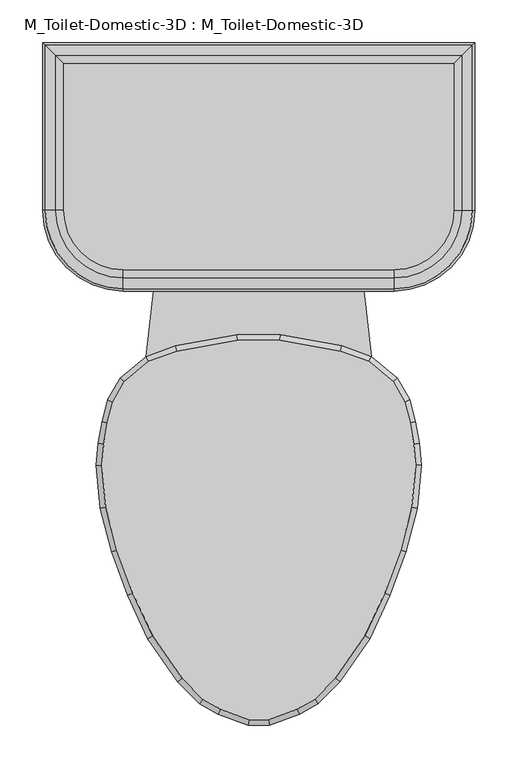
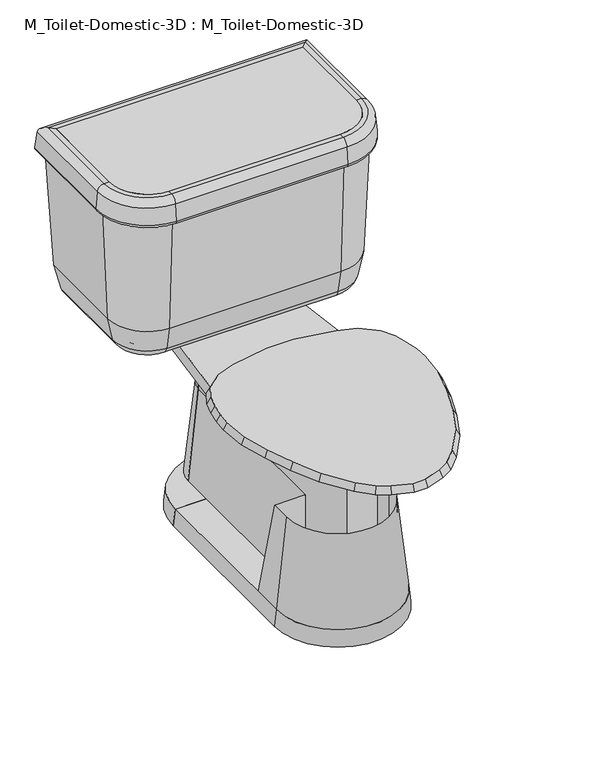
"""IFC4 building model written with IfcOpenShell, lengths in millimetres: flow terminal geometry, M_Toilet-Domestic-3D : M_Toilet-Domestic-3D."""

from ifc_helpers import new_model, si_unit, point, frame, frame_2d, origin, place, context, project, spatial, polyline, circle_curve, ellipse_curve, trimmed, segment, composite_curve, outline, extrude, faceted_brep, source, transform, mapped, element, save
from ifc_brep_helpers import plane_surface, cylinder_surface, revolved_surface, advanced_brep


def m_toilet_domestic_3d_m_toilet_domestic_3d_5cb52bd4(model_context):
    return source(origin(), model_context, "Body", "SolidModel", [
        advanced_brep(
        [(-117.7636364, 285.75, 0.0), (-38.1, 285.75, 0.0), (-38.1, 285.75, 31.75), (-114.3, 285.75, 31.75), (117.7636364, 285.75, 0.0), (114.3, 285.75, 31.75), (38.1, 285.75, 31.75), (38.1, 285.75, 0.0)],
        [
            (0, 1),
            (1, 2),
            (2, 3),
            (3, 0),
            (4, 5),
            (5, 6),
            (6, 7),
            (7, 4),
            (7, 1, circle_curve(frame((0.0, 285.75, 0.0), z_axis=(0.0, 0.0, 1.0), x_axis=(-1.0, 0.0, 0.0)), 38.1)),
            (0, 4, circle_curve(frame((0.0, 285.75, 0.0), z_axis=(0.0, 0.0, -1.0), x_axis=(-1.0, 0.0, 0.0)), 117.7636364)),
            (6, 2, circle_curve(frame((0.0, 285.75, 31.75), z_axis=(0.0, 0.0, 1.0), x_axis=(-1.0, 0.0, 0.0)), 38.1)),
            (5, 3, circle_curve(frame((0.0, 285.75, 31.75), z_axis=(0.0, 0.0, 1.0), x_axis=(-1.0, 0.0, 0.0)), 114.3)),
        ],
        [
            plane_surface(frame((0.0, 285.75, -304.8), z_axis=(0.0, -1.0, 0.0), x_axis=(-1.0, 0.0, 0.0))),
            plane_surface(frame((0.0, 285.75, -304.8), z_axis=(0.0, -1.0, 0.0), x_axis=(1.0, 0.0, 0.0))),
            plane_surface(frame((0.0, 285.75, 0.0), z_axis=(0.0, 0.0, -1.0), x_axis=(-1.0, 0.0, 0.0))),
            revolved_surface(polyline([(-38.1, 285.75, 0.0), (-38.1, 285.75, 31.75)]), (0.0, 285.75, -304.8), (0.0, 0.0, -1.0)),
            plane_surface(frame((0.0, 285.75, 31.75), z_axis=(0.0, 0.0, 1.0), x_axis=(-1.0, 0.0, 0.0))),
            revolved_surface(polyline([(-114.3, 285.75, 31.75), (-117.7636364, 285.75, 0.0)]), (0.0, 285.75, -304.8), (0.0, 0.0, -1.0)),
        ],
        [
            (0, [[1, 2, 3, 4]]),
            (1, [[5, 6, 7, 8]]),
            (2, [[9, -1, 10, -8]]),
            (3, [[11, -2, -9, -7]]),
            (4, [[12, -3, -11, -6]]),
            (5, [[-10, -4, -12, -5]]),
        ],
    ),
        advanced_brep(
        [(-38.1, 342.9, 206.375), (-57.15, 342.9, 31.75), (-38.1, 342.9, 31.75), (38.1, 342.9, 206.375), (38.1, 342.9, 31.75), (57.15, 342.9, 31.75)],
        [
            (0, 1),
            (1, 2),
            (2, 0),
            (3, 4),
            (4, 5),
            (5, 3),
            (5, 1, circle_curve(frame((0.0, 342.9, 31.75), z_axis=(0.0, 0.0, 1.0), x_axis=(-1.0, 0.0, 0.0)), 57.15)),
            (0, 3, circle_curve(frame((0.0, 342.9, 206.375), z_axis=(0.0, 0.0, -1.0), x_axis=(-1.0, 0.0, 0.0)), 38.1)),
            (4, 2, circle_curve(frame((0.0, 342.9, 31.75), z_axis=(0.0, 0.0, 1.0), x_axis=(-1.0, 0.0, 0.0)), 38.1)),
        ],
        [
            plane_surface(frame((0.0, 342.9, 31.75), z_axis=(0.0, -1.0, 0.0), x_axis=(-1.0, 0.0, 0.0))),
            plane_surface(frame((0.0, 342.9, 31.75), z_axis=(0.0, -1.0, 0.0), x_axis=(1.0, 0.0, 0.0))),
            revolved_surface(polyline([(-38.1, 342.9, 206.375), (-57.15, 342.9, 31.75)]), (0.0, 342.9, 31.75), (0.0, 0.0, -1.0)),
            plane_surface(frame((0.0, 342.9, 31.75), z_axis=(0.0, 0.0, -1.0), x_axis=(-1.0, 0.0, 0.0))),
            revolved_surface(polyline([(-38.1, 342.9, 31.75), (-38.1, 342.9, 206.375)]), (0.0, 342.9, 31.75), (0.0, 0.0, -1.0)),
        ],
        [
            (0, [[1, 2, 3]]),
            (1, [[4, 5, 6]]),
            (2, [[7, -1, 8, -6]]),
            (3, [[9, -2, -7, -5]]),
            (4, [[-8, -3, -9, -4]]),
        ],
    ),
        faceted_brep([(-157.6293435, 97.472128, 400.05), (-171.060664, 73.773864, 400.05), (-177.5851102, 49.4242991, 400.05), (-181.9845715, 24.4737144, 400.05), (-184.125744, 0.0, 400.05), (-179.7950716, -49.4998127, 400.05), (-166.347, -99.688699, 400.05), (-148.0469602, -149.9676451, 400.05), (-124.7045808, -200.0255393, 400.05), (-90.0971582, -249.9125941, 400.05), (-65.691017, -274.3187354, 400.05), (-44.8990862, -286.3229622, 400.05), (-11.5803237, -298.45, 400.05), (11.5803237, -298.45, 400.05), (44.8990862, -286.3229622, 400.05), (65.691017, -274.3187354, 400.05), (90.0971582, -249.9125941, 400.05), (124.7045808, -200.0255393, 400.05), (148.0469602, -149.9676451, 400.05), (166.347, -99.688699, 400.05), (179.7950716, -49.4998127, 400.05), (184.125744, 0.0, 400.05), (181.9845715, 24.4737144, 400.05), (177.5851102, 49.4242991, 400.05), (171.060664, 73.773864, 400.05), (157.6293435, 97.472128, 400.05), (129.0942628, 121.4159037, 400.05), (95.7755003, 133.5429415, 400.05), (24.844447, 146.05, 400.05), (-24.844447, 146.05, 400.05), (-95.7755003, 133.5429415, 400.05), (-129.0942628, 121.4159037, 400.05), (-162.5887836, 101.6, 387.2181453), (-132.3182423, 127.0, 387.2181453), (-97.4252791, 139.7, 387.2181453), (-25.4, 152.4, 387.2181453), (25.4, 152.4, 387.2181453), (97.4252791, 139.7, 387.2181453), (132.3182423, 127.0, 387.2181453), (162.5887836, 101.6, 387.2181453), (176.9845865, 76.2, 387.2181453), (183.790496, 50.8, 387.2181453), (188.2862441, 25.3033453, 387.2181453), (190.5, 0.0, 387.2181453), (186.0724883, -50.6066907, 387.2181453), (172.4088722, -101.6, 387.2181453), (153.9191843, -152.4, 387.2181453), (130.2307553, -203.2, 387.2181453), (94.9900085, -254.0, 387.2181453), (69.5900085, -279.4, 387.2181453), (47.5929632, -292.1, 387.2181453), (12.7, -304.8, 387.2181453), (-12.7, -304.8, 387.2181453), (-47.5929632, -292.1, 387.2181453), (-69.5900085, -279.4, 387.2181453), (-94.9900085, -254.0, 387.2181453), (-130.2307553, -203.2, 387.2181453), (-153.9191843, -152.4, 387.2181453), (-172.4088722, -101.6, 387.2181453), (-186.0724883, -50.6066907, 387.2181453), (-190.5, 0.0, 387.2181453), (-188.2862441, 25.3033453, 387.2181453), (-183.790496, 50.8, 387.2181453), (-176.9845865, 76.2, 387.2181453)], [[[0, 1, 2, 3, 4, 5, 6, 7, 8, 9, 10, 11, 12, 13, 14, 15, 16, 17, 18, 19, 20, 21, 22, 23, 24, 25, 26, 27, 28, 29, 30, 31]], [[32, 33, 34, 35, 36, 37, 38, 39, 40, 41, 42, 43, 44, 45, 46, 47, 48, 49, 50, 51, 52, 53, 54, 55, 56, 57, 58, 59, 60, 61, 62, 63]], [[32, 63, 1, 0]], [[63, 62, 2, 1]], [[62, 61, 3, 2]], [[61, 60, 4, 3]], [[60, 59, 5, 4]], [[59, 58, 6, 5]], [[58, 57, 7, 6]], [[57, 56, 8, 7]], [[56, 55, 9, 8]], [[55, 54, 10, 9]], [[54, 53, 11, 10]], [[53, 52, 12, 11]], [[52, 51, 13, 12]], [[51, 50, 14, 13]], [[50, 49, 15, 14]], [[49, 48, 16, 15]], [[48, 47, 17, 16]], [[47, 46, 18, 17]], [[46, 45, 19, 18]], [[45, 44, 20, 19]], [[44, 43, 21, 20]], [[43, 42, 22, 21]], [[42, 41, 23, 22]], [[41, 40, 24, 23]], [[40, 39, 25, 24]], [[39, 38, 26, 25]], [[38, 37, 27, 26]], [[37, 36, 28, 27]], [[36, 35, 29, 28]], [[35, 34, 30, 29]], [[34, 33, 31, 30]], [[33, 32, 0, 31]]]),
        extrude(outline(composite_curve([segment(polyline([(228.5868869, 469.8868869), (228.5868869, 298.45)]), True, "CONTINUOUS"), segment(trimmed(circle_curve(frame_2d((158.75, 298.45)), 69.8368869), [point((228.5868869, 298.45))], [point((158.75, 228.6131131))], False, "CARTESIAN"), True, "CONTINUOUS"), segment(polyline([(158.75, 228.6131131), (-158.75, 228.6131131)]), True, "CONTINUOUS"), segment(trimmed(circle_curve(frame_2d((-158.75, 298.45)), 69.8368869), [point((-158.75, 228.6131131))], [point((-228.5868869, 298.45))], False, "CARTESIAN"), True, "CONTINUOUS"), segment(polyline([(-228.5868869, 298.45), (-228.5868869, 469.8868869), (228.5868869, 469.8868869)]), True, "CONTINUOUS")], self_intersect=False)), frame((0.0, 0.0, 654.05), z_axis=(0.0, 0.0, 1.0), x_axis=(1.0, 0.0, 0.0)), (0.0, 0.0, 1.0), 50.8),
        extrude(outline(composite_curve([segment(trimmed(circle_curve(frame_2d((0.0, 342.9)), 38.1), [point((-38.1, 342.9))], [point((38.1, 342.9))], False, "CARTESIAN"), True, "CONTINUOUS"), segment(polyline([(38.1, 342.9), (-38.1, 342.9)]), True, "CONTINUOUS")], self_intersect=False)), frame((0.0, 0.0, 206.375), z_axis=(0.0, 0.0, 1.0), x_axis=(1.0, 0.0, 0.0)), (0.0, 0.0, 1.0), 130.175),
        advanced_brep(
        [(177.8, 419.1, 387.2181453), (177.8, 419.1, 374.65), (177.8, 298.45, 374.65), (177.8, 298.45, 387.2181453), (192.8020829, 434.1020829, 387.2181453), (192.8020829, 298.45, 387.2181453), (211.4650931, 452.7650931, 402.4478636), (211.4650931, 298.45, 402.4478636), (218.7732506, 460.0732506, 438.15), (218.7732506, 298.45, 438.15), (228.5868869, 469.8868869, 654.05), (228.5868869, 298.45, 654.05), (228.5868869, 469.8868869, 704.85), (228.5868869, 298.45, 704.85), (237.91817, 479.21817, 704.85), (237.91817, 298.45, 704.85), (250.5698426, 491.8698426, 693.2568779), (250.5698426, 298.45, 693.2568779), (253.3960274, 494.6960274, 660.953439), (253.3960274, 298.45, 660.953439), (247.070191, 488.370191, 654.05), (247.070191, 298.45, 654.05), (241.3, 482.6, 654.05), (241.3, 298.45, 654.05), (231.4863636, 472.7863636, 438.15), (231.4863636, 298.45, 438.15), (222.3416824, 463.6416824, 393.4759963), (222.3416824, 298.45, 393.4759963), (197.8071664, 439.1071664, 374.65), (197.8071664, 298.45, 374.65), (158.75, 279.4, 387.2181453), (158.75, 279.4, 374.65), (158.75, 264.3979171, 387.2181453), (158.75, 245.7349069, 402.4478636), (158.75, 238.4267494, 438.15), (158.75, 228.6131131, 654.05), (158.75, 228.6131131, 704.85), (158.75, 219.28183, 704.85), (158.75, 206.6301574, 693.2568779), (158.75, 203.8039726, 660.953439), (158.75, 210.129809, 654.05), (158.75, 215.9, 654.05), (158.75, 225.7136364, 438.15), (158.75, 234.8583176, 393.4759963), (158.75, 259.3928336, 374.65), (-158.75, 279.4, 374.65), (-158.75, 279.4, 387.2181453), (-158.75, 264.3979171, 387.2181453), (-158.75, 245.7349069, 402.4478636), (-158.75, 238.4267494, 438.15), (-158.75, 228.6131131, 654.05), (-158.75, 228.6131131, 704.85), (-158.75, 219.28183, 704.85), (-158.75, 206.6301574, 693.2568779), (-158.75, 203.8039726, 660.953439), (-158.75, 210.129809, 654.05), (-158.75, 215.9, 654.05), (-158.75, 225.7136364, 438.15), (-158.75, 234.8583176, 393.4759963), (-158.75, 259.3928336, 374.65), (-177.8, 298.45, 387.2181453), (-177.8, 298.45, 374.65), (-192.8020829, 298.45, 387.2181453), (-211.4650931, 298.45, 402.4478636), (-218.7732506, 298.45, 438.15), (-228.5868869, 298.45, 654.05), (-228.5868869, 298.45, 704.85), (-237.91817, 298.45, 704.85), (-250.5698426, 298.45, 693.2568779), (-253.3960274, 298.45, 660.953439), (-247.070191, 298.45, 654.05), (-241.3, 298.45, 654.05), (-231.4863636, 298.45, 438.15), (-222.3416824, 298.45, 393.4759963), (-197.8071664, 298.45, 374.65), (-177.8, 419.1, 374.65), (-177.8, 419.1, 387.2181453), (-192.8020829, 434.1020829, 387.2181453), (-211.4650931, 452.7650931, 402.4478636), (-218.7732506, 460.0732506, 438.15), (-228.5868869, 469.8868869, 654.05), (-228.5868869, 469.8868869, 704.85), (-237.91817, 479.21817, 704.85), (-250.5698426, 491.8698426, 693.2568779), (-253.3960274, 494.6960274, 660.953439), (-247.070191, 488.370191, 654.05), (-241.3, 482.6, 654.05), (-231.4863636, 472.7863636, 438.15), (-222.3416824, 463.6416824, 393.4759963), (-197.8071664, 439.1071664, 374.65)],
        [
            (0, 1),
            (1, 2),
            (2, 3),
            (3, 0),
            (4, 0),
            (3, 5),
            (5, 4),
            (6, 4, ellipse_curve(frame((192.8020829, 434.1020829, 406.2681453), z_axis=(-0.7071067811865451, 0.7071067811865498, 0.0), x_axis=(-0.7071067811865497, -0.7071067811865452, 0.0)), 26.9407684, 19.05)),
            (5, 7, circle_curve(frame((192.8020829, 298.45, 406.2681453), z_axis=(0.0, -1.0, 0.0), x_axis=(1.0, 0.0, 0.0)), 19.05)),
            (7, 6),
            (8, 6),
            (7, 9),
            (9, 8),
            (10, 8),
            (9, 11),
            (11, 10),
            (12, 10),
            (11, 13),
            (13, 12),
            (14, 12),
            (13, 15),
            (15, 14),
            (16, 14, ellipse_curve(frame((237.91817, 479.21817, 692.15), z_axis=(0.7071067811865451, -0.7071067811865498, 0.0), x_axis=(0.7071067811865497, 0.7071067811865452, 0.0)), 17.9605122, 12.7)),
            (15, 17, circle_curve(frame((237.91817, 298.45, 692.15), z_axis=(0.0, 1.0, 0.0), x_axis=(1.0, 0.0, 0.0)), 12.7)),
            (17, 16),
            (18, 16),
            (17, 19),
            (19, 18),
            (20, 18, ellipse_curve(frame((247.070191, 488.370191, 660.4), z_axis=(0.7071067811865451, -0.7071067811865498, 0.0), x_axis=(0.7071067811865497, 0.7071067811865452, 0.0)), 8.9802561, 6.35)),
            (19, 21, circle_curve(frame((247.070191, 298.45, 660.4), z_axis=(0.0, 1.0, 0.0), x_axis=(1.0, 0.0, 0.0)), 6.35)),
            (21, 20),
            (22, 20),
            (21, 23),
            (23, 22),
            (24, 22),
            (23, 25),
            (25, 24),
            (26, 24),
            (25, 27),
            (27, 26),
            (28, 26, ellipse_curve(frame((197.8071664, 439.1071664, 400.05), z_axis=(0.7071067811865451, -0.7071067811865498, 0.0), x_axis=(0.7071067811865497, 0.7071067811865452, 0.0)), 35.9210245, 25.4)),
            (27, 29, circle_curve(frame((197.8071664, 298.45, 400.05), z_axis=(0.0, 1.0, 0.0), x_axis=(1.0, 0.0, 0.0)), 25.4)),
            (29, 28),
            (1, 28),
            (29, 2),
            (30, 3, circle_curve(frame((158.75, 298.45, 387.2181453), z_axis=(0.0, 0.0, 1.0), x_axis=(1.0, 0.0, 0.0)), 19.05)),
            (2, 31, circle_curve(frame((158.75, 298.45, 374.65), z_axis=(0.0, 0.0, -1.0), x_axis=(1.0, 0.0, 0.0)), 19.05)),
            (31, 30),
            (32, 5, circle_curve(frame((158.75, 298.45, 387.2181453), z_axis=(0.0, 0.0, 1.0), x_axis=(1.0, 0.0, 0.0)), 34.0520829)),
            (30, 32),
            (33, 7, circle_curve(frame((158.75, 298.45, 402.4478636), z_axis=(0.0, 0.0, 1.0), x_axis=(1.0, 0.0, 0.0)), 52.7150931)),
            (32, 33, circle_curve(frame((158.75, 264.3979171, 406.2681453), z_axis=(-1.0, 0.0, 0.0), x_axis=(0.0, -1.0, 0.0)), 19.05)),
            (34, 9, circle_curve(frame((158.75, 298.45, 438.15), z_axis=(0.0, 0.0, 1.0), x_axis=(1.0, 0.0, 0.0)), 60.0232506)),
            (33, 34),
            (35, 11, circle_curve(frame((158.75, 298.45, 654.05), z_axis=(0.0, 0.0, 1.0), x_axis=(1.0, 0.0, 0.0)), 69.8368869)),
            (34, 35),
            (36, 13, circle_curve(frame((158.75, 298.45, 704.85), z_axis=(0.0, 0.0, 1.0), x_axis=(1.0, 0.0, 0.0)), 69.8368869)),
            (35, 36),
            (37, 15, circle_curve(frame((158.75, 298.45, 704.85), z_axis=(0.0, 0.0, 1.0), x_axis=(1.0, 0.0, 0.0)), 79.16817)),
            (36, 37),
            (38, 17, circle_curve(frame((158.75, 298.45, 693.2568779), z_axis=(0.0, 0.0, 1.0), x_axis=(1.0, 0.0, 0.0)), 91.8198426)),
            (37, 38, circle_curve(frame((158.75, 219.28183, 692.15), z_axis=(1.0, 0.0, 0.0), x_axis=(0.0, -1.0, 0.0)), 12.7)),
            (39, 19, circle_curve(frame((158.75, 298.45, 660.953439), z_axis=(0.0, 0.0, 1.0), x_axis=(1.0, 0.0, 0.0)), 94.6460274)),
            (38, 39),
            (40, 21, circle_curve(frame((158.75, 298.45, 654.05), z_axis=(0.0, 0.0, 1.0), x_axis=(1.0, 0.0, 0.0)), 88.320191)),
            (39, 40, circle_curve(frame((158.75, 210.129809, 660.4), z_axis=(1.0, 0.0, 0.0), x_axis=(0.0, -1.0, 0.0)), 6.35)),
            (41, 23, circle_curve(frame((158.75, 298.45, 654.05), z_axis=(0.0, 0.0, 1.0), x_axis=(1.0, 0.0, 0.0)), 82.55)),
            (40, 41),
            (42, 25, circle_curve(frame((158.75, 298.45, 438.15), z_axis=(0.0, 0.0, 1.0), x_axis=(1.0, 0.0, 0.0)), 72.7363636)),
            (41, 42),
            (43, 27, circle_curve(frame((158.75, 298.45, 393.4759963), z_axis=(0.0, 0.0, 1.0), x_axis=(1.0, 0.0, 0.0)), 63.5916824)),
            (42, 43),
            (44, 29, circle_curve(frame((158.75, 298.45, 374.65), z_axis=(0.0, 0.0, 1.0), x_axis=(1.0, 0.0, 0.0)), 39.0571664)),
            (43, 44, circle_curve(frame((158.75, 259.3928336, 400.05), z_axis=(1.0, 0.0, 0.0), x_axis=(0.0, -1.0, 0.0)), 25.4)),
            (44, 31),
            (31, 45),
            (45, 46),
            (46, 30),
            (46, 47),
            (47, 32),
            (47, 48, circle_curve(frame((-158.75, 264.3979171, 406.2681453), z_axis=(-1.0, 0.0, 0.0), x_axis=(0.0, -1.0, 0.0)), 19.05)),
            (48, 33),
            (48, 49),
            (49, 34),
            (49, 50),
            (50, 35),
            (50, 51),
            (51, 36),
            (51, 52),
            (52, 37),
            (52, 53, circle_curve(frame((-158.75, 219.28183, 692.15), z_axis=(1.0, 0.0, 0.0), x_axis=(0.0, -1.0, 0.0)), 12.7)),
            (53, 38),
            (53, 54),
            (54, 39),
            (54, 55, circle_curve(frame((-158.75, 210.129809, 660.4), z_axis=(1.0, 0.0, 0.0), x_axis=(0.0, -1.0, 0.0)), 6.35)),
            (55, 40),
            (55, 56),
            (56, 41),
            (56, 57),
            (57, 42),
            (57, 58),
            (58, 43),
            (58, 59, circle_curve(frame((-158.75, 259.3928336, 400.05), z_axis=(1.0, 0.0, 0.0), x_axis=(0.0, -1.0, 0.0)), 25.4)),
            (59, 44),
            (59, 45),
            (60, 46, circle_curve(frame((-158.75, 298.45, 387.2181453), z_axis=(0.0, 0.0, 1.0), x_axis=(0.0, -1.0, 0.0)), 19.05)),
            (45, 61, circle_curve(frame((-158.75, 298.45, 374.65), z_axis=(0.0, 0.0, -1.0), x_axis=(0.0, -1.0, 0.0)), 19.05)),
            (61, 60),
            (62, 47, circle_curve(frame((-158.75, 298.45, 387.2181453), z_axis=(0.0, 0.0, 1.0), x_axis=(0.0, -1.0, 0.0)), 34.0520829)),
            (60, 62),
            (63, 48, circle_curve(frame((-158.75, 298.45, 402.4478636), z_axis=(0.0, 0.0, 1.0), x_axis=(0.0, -1.0, 0.0)), 52.7150931)),
            (62, 63, circle_curve(frame((-192.8020829, 298.45, 406.2681453), z_axis=(0.0, 1.0, 0.0), x_axis=(-1.0, 0.0, 0.0)), 19.05)),
            (64, 49, circle_curve(frame((-158.75, 298.45, 438.15), z_axis=(0.0, 0.0, 1.0), x_axis=(0.0, -1.0, 0.0)), 60.0232506)),
            (63, 64),
            (65, 50, circle_curve(frame((-158.75, 298.45, 654.05), z_axis=(0.0, 0.0, 1.0), x_axis=(0.0, -1.0, 0.0)), 69.8368869)),
            (64, 65),
            (66, 51, circle_curve(frame((-158.75, 298.45, 704.85), z_axis=(0.0, 0.0, 1.0), x_axis=(0.0, -1.0, 0.0)), 69.8368869)),
            (65, 66),
            (67, 52, circle_curve(frame((-158.75, 298.45, 704.85), z_axis=(0.0, 0.0, 1.0), x_axis=(0.0, -1.0, 0.0)), 79.16817)),
            (66, 67),
            (68, 53, circle_curve(frame((-158.75, 298.45, 693.2568779), z_axis=(0.0, 0.0, 1.0), x_axis=(0.0, -1.0, 0.0)), 91.8198426)),
            (67, 68, circle_curve(frame((-237.91817, 298.45, 692.15), z_axis=(0.0, -1.0, 0.0), x_axis=(-1.0, 0.0, 0.0)), 12.7)),
            (69, 54, circle_curve(frame((-158.75, 298.45, 660.953439), z_axis=(0.0, 0.0, 1.0), x_axis=(0.0, -1.0, 0.0)), 94.6460274)),
            (68, 69),
            (70, 55, circle_curve(frame((-158.75, 298.45, 654.05), z_axis=(0.0, 0.0, 1.0), x_axis=(0.0, -1.0, 0.0)), 88.320191)),
            (69, 70, circle_curve(frame((-247.070191, 298.45, 660.4), z_axis=(0.0, -1.0, 0.0), x_axis=(-1.0, 0.0, 0.0)), 6.35)),
            (71, 56, circle_curve(frame((-158.75, 298.45, 654.05), z_axis=(0.0, 0.0, 1.0), x_axis=(0.0, -1.0, 0.0)), 82.55)),
            (70, 71),
            (72, 57, circle_curve(frame((-158.75, 298.45, 438.15), z_axis=(0.0, 0.0, 1.0), x_axis=(0.0, -1.0, 0.0)), 72.7363636)),
            (71, 72),
            (73, 58, circle_curve(frame((-158.75, 298.45, 393.4759963), z_axis=(0.0, 0.0, 1.0), x_axis=(0.0, -1.0, 0.0)), 63.5916824)),
            (72, 73),
            (74, 59, circle_curve(frame((-158.75, 298.45, 374.65), z_axis=(0.0, 0.0, 1.0), x_axis=(0.0, -1.0, 0.0)), 39.0571664)),
            (73, 74, circle_curve(frame((-197.8071664, 298.45, 400.05), z_axis=(0.0, -1.0, 0.0), x_axis=(-1.0, 0.0, 0.0)), 25.4)),
            (74, 61),
            (61, 75),
            (75, 76),
            (76, 60),
            (76, 77),
            (77, 62),
            (77, 78, ellipse_curve(frame((-192.8020829, 434.1020829, 406.2681453), z_axis=(0.7071067811865498, 0.7071067811865451, 0.0), x_axis=(-0.7071067811865451, 0.70710678118655, 0.0)), 26.9407684, 19.05)),
            (78, 63),
            (78, 79),
            (79, 64),
            (79, 80),
            (80, 65),
            (80, 81),
            (81, 66),
            (81, 82),
            (82, 67),
            (82, 83, ellipse_curve(frame((-237.91817, 479.21817, 692.15), z_axis=(-0.7071067811865498, -0.7071067811865451, 0.0), x_axis=(0.7071067811865451, -0.70710678118655, 0.0)), 17.9605122, 12.7)),
            (83, 68),
            (83, 84),
            (84, 69),
            (84, 85, ellipse_curve(frame((-247.070191, 488.370191, 660.4), z_axis=(-0.7071067811865498, -0.7071067811865451, 0.0), x_axis=(0.7071067811865451, -0.70710678118655, 0.0)), 8.9802561, 6.35)),
            (85, 70),
            (85, 86),
            (86, 71),
            (86, 87),
            (87, 72),
            (87, 88),
            (88, 73),
            (88, 89, ellipse_curve(frame((-197.8071664, 439.1071664, 400.05), z_axis=(-0.7071067811865498, -0.7071067811865451, 0.0), x_axis=(0.7071067811865451, -0.70710678118655, 0.0)), 35.9210245, 25.4)),
            (89, 74),
            (89, 75),
            (75, 1),
            (0, 76),
            (4, 77),
            (6, 78),
            (8, 79),
            (10, 80),
            (12, 81),
            (14, 82),
            (16, 83),
            (18, 84),
            (20, 85),
            (22, 86),
            (24, 87),
            (26, 88),
            (28, 89),
        ],
        [
            plane_surface(frame((177.8, 419.1, 374.65), z_axis=(-1.0, 0.0, 0.0), x_axis=(0.0, -1.0, 0.0))),
            plane_surface(frame((177.8, 419.1, 387.2181453), z_axis=(0.0, 0.0, 1.0), x_axis=(0.0, -1.0, 0.0))),
            revolved_surface(polyline([(211.8520829, 298.45, 406.2681453), (211.8520829, 453.1520829260162, 406.2681453)]), (192.8020829, 419.1, 406.2681453), (0.0, -1.0, 0.0)),
            plane_surface(frame((211.4650931, 452.7650931, 402.4478636), z_axis=(-0.9796855721787505, 0.0, 0.2005397209153197), x_axis=(0.0, -1.0, 0.0))),
            plane_surface(frame((218.7732506, 460.0732506, 438.15), z_axis=(-0.9989685402102993, 0.0, 0.04540766091865541), x_axis=(0.0, -1.0, 0.0))),
            plane_surface(frame((228.5868869, 469.8868869, 654.05), z_axis=(-1.0, 0.0, 0.0), x_axis=(0.0, -1.0, 0.0))),
            plane_surface(frame((228.5868869, 469.8868869, 704.85), z_axis=(0.0, 0.0, 1.0), x_axis=(0.0, -1.0, 0.0))),
            cylinder_surface(frame((237.91817, 419.1, 692.15), z_axis=(0.0, 1.0, 0.0), x_axis=(1.0, 0.0, 0.0)), 12.7),
            plane_surface(frame((250.5698426, 491.8698426, 693.2568779), z_axis=(0.9961946980917448, 0.0, 0.08715574274766702), x_axis=(0.0, -1.0, 0.0))),
            cylinder_surface(frame((247.070191, 419.1, 660.4), z_axis=(0.0, 1.0, 0.0), x_axis=(1.0, 0.0, 0.0)), 6.35),
            plane_surface(frame((247.070191, 488.370191, 654.05), z_axis=(0.0, 0.0, -1.0), x_axis=(0.0, -1.0, 0.0))),
            plane_surface(frame((241.3, 482.6, 654.05), z_axis=(0.9989685402102995, 0.0, -0.04540766091865437), x_axis=(0.0, -1.0, 0.0))),
            plane_surface(frame((231.4863636, 472.7863636, 438.15), z_axis=(0.9796855721787479, 0.0, -0.2005397209153326), x_axis=(0.0, -1.0, 0.0))),
            cylinder_surface(frame((197.8071664, 419.1, 400.05), z_axis=(0.0, 1.0, 0.0), x_axis=(1.0, 0.0, 0.0)), 25.4),
            plane_surface(frame((197.8071664, 439.1071664, 374.65), z_axis=(0.0, 0.0, -1.0), x_axis=(0.0, -1.0, 0.0))),
            revolved_surface(polyline([(177.8, 298.45, 374.65), (177.8, 298.45, 387.2181453)]), (158.75, 298.45, 0.0), (0.0, 0.0, -1.0)),
            plane_surface(frame((158.75, 298.45, 387.2181453), z_axis=(0.0, 0.0, 1.0), x_axis=(1.0, 0.0, 0.0))),
            revolved_surface(trimmed(ellipse_curve(frame((192.8020829, 298.45, 406.2681453), z_axis=(0.0, -1.0, 0.0), x_axis=(1.0, 0.0, 0.0)), 19.05, 19.05), [point((192.8020829, 298.45, 387.2181453))], [point((211.4650931, 298.45, 402.4478636))], True, "CARTESIAN"), (158.75, 298.45, 0.0), (0.0, 0.0, -1.0)),
            revolved_surface(polyline([(211.4650931, 298.45, 402.4478636), (218.7732506, 298.45, 438.15)]), (158.75, 298.45, 0.0), (0.0, 0.0, -1.0)),
            revolved_surface(polyline([(218.7732506, 298.45, 438.15), (228.5868869, 298.45, 654.05)]), (158.75, 298.45, 0.0), (0.0, 0.0, -1.0)),
            revolved_surface(polyline([(228.5868869, 298.45, 654.05), (228.5868869, 298.45, 704.85)]), (158.75, 298.45, 0.0), (0.0, 0.0, -1.0)),
            plane_surface(frame((158.75, 298.45, 704.85), z_axis=(0.0, 0.0, 1.0), x_axis=(1.0, 0.0, 0.0))),
            revolved_surface(trimmed(ellipse_curve(frame((237.91817, 298.45, 692.15), z_axis=(0.0, 1.0, 0.0), x_axis=(1.0, 0.0, 0.0)), 12.7, 12.7), [point((237.91817, 298.45, 704.85))], [point((250.5698426, 298.45, 693.2568779))], True, "CARTESIAN"), (158.75, 298.45, 0.0), (0.0, 0.0, -1.0)),
            revolved_surface(polyline([(250.5698426, 298.45, 693.2568779), (253.3960274, 298.45, 660.953439)]), (158.75, 298.45, 0.0), (0.0, 0.0, -1.0)),
            revolved_surface(trimmed(ellipse_curve(frame((247.070191, 298.45, 660.4), z_axis=(0.0, 1.0, 0.0), x_axis=(1.0, 0.0, 0.0)), 6.35, 6.35), [point((253.3960274, 298.45, 660.953439))], [point((247.070191, 298.45, 654.05))], True, "CARTESIAN"), (158.75, 298.45, 0.0), (0.0, 0.0, -1.0)),
            plane_surface(frame((158.75, 298.45, 654.05), z_axis=(0.0, 0.0, -1.0), x_axis=(1.0, 0.0, 0.0))),
            revolved_surface(polyline([(241.3, 298.45, 654.05), (231.4863636, 298.45, 438.15)]), (158.75, 298.45, 0.0), (0.0, 0.0, -1.0)),
            revolved_surface(polyline([(231.4863636, 298.45, 438.15), (222.3416824, 298.45, 393.4759963)]), (158.75, 298.45, 0.0), (0.0, 0.0, -1.0)),
            revolved_surface(trimmed(ellipse_curve(frame((197.8071664, 298.45, 400.05), z_axis=(0.0, 1.0, 0.0), x_axis=(1.0, 0.0, 0.0)), 25.4, 25.4), [point((222.3416824, 298.45, 393.4759963))], [point((197.8071664, 298.45, 374.65))], True, "CARTESIAN"), (158.75, 298.45, 0.0), (0.0, 0.0, -1.0)),
            plane_surface(frame((158.75, 298.45, 374.65), z_axis=(0.0, 0.0, -1.0), x_axis=(1.0, 0.0, 0.0))),
            plane_surface(frame((158.75, 279.4, 374.65), z_axis=(0.0, 1.0, 0.0), x_axis=(-1.0, 0.0, 0.0))),
            plane_surface(frame((158.75, 279.4, 387.2181453), z_axis=(0.0, 0.0, 1.0), x_axis=(-1.0, 0.0, 0.0))),
            revolved_surface(polyline([(-158.75, 245.34791709999996, 406.2681453), (158.75, 245.34791709999996, 406.2681453)]), (158.75, 264.3979171, 406.2681453), (-1.0, 0.0, 0.0)),
            plane_surface(frame((158.75, 245.7349069, 402.4478636), z_axis=(0.0, 0.9796855721787505, 0.2005397209153197), x_axis=(-1.0, 0.0, 0.0))),
            plane_surface(frame((158.75, 238.4267494, 438.15), z_axis=(0.0, 0.9989685402102993, 0.04540766091865541), x_axis=(-1.0, 0.0, 0.0))),
            plane_surface(frame((158.75, 228.6131131, 654.05), z_axis=(0.0, 1.0, 0.0), x_axis=(-1.0, 0.0, 0.0))),
            plane_surface(frame((158.75, 228.6131131, 704.85), z_axis=(0.0, 0.0, 1.0), x_axis=(-1.0, 0.0, 0.0))),
            cylinder_surface(frame((158.75, 219.28183, 692.15), z_axis=(1.0, 0.0, 0.0), x_axis=(0.0, -1.0, 0.0)), 12.7),
            plane_surface(frame((158.75, 206.6301574, 693.2568779), z_axis=(0.0, -0.9961946980917448, 0.08715574274766702), x_axis=(-1.0, 0.0, 0.0))),
            cylinder_surface(frame((158.75, 210.129809, 660.4), z_axis=(1.0, 0.0, 0.0), x_axis=(0.0, -1.0, 0.0)), 6.35),
            plane_surface(frame((158.75, 210.129809, 654.05), z_axis=(0.0, 0.0, -1.0), x_axis=(-1.0, 0.0, 0.0))),
            plane_surface(frame((158.75, 215.9, 654.05), z_axis=(0.0, -0.9989685402102995, -0.04540766091865437), x_axis=(-1.0, 0.0, 0.0))),
            plane_surface(frame((158.75, 225.7136364, 438.15), z_axis=(0.0, -0.9796855721787479, -0.2005397209153326), x_axis=(-1.0, 0.0, 0.0))),
            cylinder_surface(frame((158.75, 259.3928336, 400.05), z_axis=(1.0, 0.0, 0.0), x_axis=(0.0, -1.0, 0.0)), 25.4),
            plane_surface(frame((158.75, 259.3928336, 374.65), z_axis=(0.0, 0.0, -1.0), x_axis=(-1.0, 0.0, 0.0))),
            revolved_surface(polyline([(-158.75, 279.4, 374.65), (-158.75, 279.4, 387.2181453)]), (-158.75, 298.45, 0.0), (0.0, 0.0, -1.0)),
            plane_surface(frame((-158.75, 298.45, 387.2181453), z_axis=(0.0, 0.0, 1.0), x_axis=(0.0, -1.0, 0.0))),
            revolved_surface(trimmed(ellipse_curve(frame((-158.75, 264.3979171, 406.2681453), z_axis=(-1.0, 0.0, 0.0), x_axis=(0.0, -1.0, 0.0)), 19.05, 19.05), [point((-158.75, 264.3979171, 387.2181453))], [point((-158.75, 245.7349069, 402.4478636))], True, "CARTESIAN"), (-158.75, 298.45, 0.0), (0.0, 0.0, -1.0)),
            revolved_surface(polyline([(-158.75, 245.7349069, 402.4478636), (-158.75, 238.4267494, 438.15)]), (-158.75, 298.45, 0.0), (0.0, 0.0, -1.0)),
            revolved_surface(polyline([(-158.75, 238.4267494, 438.15), (-158.75, 228.6131131, 654.05)]), (-158.75, 298.45, 0.0), (0.0, 0.0, -1.0)),
            revolved_surface(polyline([(-158.75, 228.6131131, 654.05), (-158.75, 228.6131131, 704.85)]), (-158.75, 298.45, 0.0), (0.0, 0.0, -1.0)),
            plane_surface(frame((-158.75, 298.45, 704.85), z_axis=(0.0, 0.0, 1.0), x_axis=(0.0, -1.0, 0.0))),
            revolved_surface(trimmed(ellipse_curve(frame((-158.75, 219.28183, 692.15), z_axis=(1.0, 0.0, 0.0), x_axis=(0.0, -1.0, 0.0)), 12.7, 12.7), [point((-158.75, 219.28183, 704.85))], [point((-158.75, 206.6301574, 693.2568779))], True, "CARTESIAN"), (-158.75, 298.45, 0.0), (0.0, 0.0, -1.0)),
            revolved_surface(polyline([(-158.75, 206.6301574, 693.2568779), (-158.75, 203.8039726, 660.953439)]), (-158.75, 298.45, 0.0), (0.0, 0.0, -1.0)),
            revolved_surface(trimmed(ellipse_curve(frame((-158.75, 210.129809, 660.4), z_axis=(1.0, 0.0, 0.0), x_axis=(0.0, -1.0, 0.0)), 6.35, 6.35), [point((-158.75, 203.8039726, 660.953439))], [point((-158.75, 210.129809, 654.05))], True, "CARTESIAN"), (-158.75, 298.45, 0.0), (0.0, 0.0, -1.0)),
            plane_surface(frame((-158.75, 298.45, 654.05), z_axis=(0.0, 0.0, -1.0), x_axis=(0.0, -1.0, 0.0))),
            revolved_surface(polyline([(-158.75, 215.9, 654.05), (-158.75, 225.7136364, 438.15)]), (-158.75, 298.45, 0.0), (0.0, 0.0, -1.0)),
            revolved_surface(polyline([(-158.75, 225.7136364, 438.15), (-158.75, 234.8583176, 393.4759963)]), (-158.75, 298.45, 0.0), (0.0, 0.0, -1.0)),
            revolved_surface(trimmed(ellipse_curve(frame((-158.75, 259.3928336, 400.05), z_axis=(1.0, 0.0, 0.0), x_axis=(0.0, -1.0, 0.0)), 25.4, 25.4), [point((-158.75, 234.8583176, 393.4759963))], [point((-158.75, 259.3928336, 374.65))], True, "CARTESIAN"), (-158.75, 298.45, 0.0), (0.0, 0.0, -1.0)),
            plane_surface(frame((-158.75, 298.45, 374.65), z_axis=(0.0, 0.0, -1.0), x_axis=(0.0, -1.0, 0.0))),
            plane_surface(frame((-177.8, 298.45, 374.65), z_axis=(1.0, 0.0, 0.0), x_axis=(0.0, 1.0, 0.0))),
            plane_surface(frame((-177.8, 298.45, 387.2181453), z_axis=(0.0, 0.0, 1.0), x_axis=(0.0, 1.0, 0.0))),
            revolved_surface(polyline([(-211.8520829, 453.15208292601636, 406.2681453), (-211.8520829, 298.45, 406.2681453)]), (-192.8020829, 298.45, 406.2681453), (0.0, 1.0, 0.0)),
            plane_surface(frame((-211.4650931, 298.45, 402.4478636), z_axis=(0.9796855721787505, 0.0, 0.2005397209153197), x_axis=(0.0, 1.0, 0.0))),
            plane_surface(frame((-218.7732506, 298.45, 438.15), z_axis=(0.9989685402102993, 0.0, 0.04540766091865541), x_axis=(0.0, 1.0, 0.0))),
            plane_surface(frame((-228.5868869, 298.45, 654.05), z_axis=(1.0, 0.0, 0.0), x_axis=(0.0, 1.0, 0.0))),
            plane_surface(frame((-228.5868869, 298.45, 704.85), z_axis=(0.0, 0.0, 1.0), x_axis=(0.0, 1.0, 0.0))),
            cylinder_surface(frame((-237.91817, 298.45, 692.15), z_axis=(0.0, -1.0, 0.0), x_axis=(-1.0, 0.0, 0.0)), 12.7),
            plane_surface(frame((-250.5698426, 298.45, 693.2568779), z_axis=(-0.9961946980917448, 0.0, 0.08715574274766702), x_axis=(0.0, 1.0, 0.0))),
            cylinder_surface(frame((-247.070191, 298.45, 660.4), z_axis=(0.0, -1.0, 0.0), x_axis=(-1.0, 0.0, 0.0)), 6.35),
            plane_surface(frame((-247.070191, 298.45, 654.05), z_axis=(0.0, 0.0, -1.0), x_axis=(0.0, 1.0, 0.0))),
            plane_surface(frame((-241.3, 298.45, 654.05), z_axis=(-0.9989685402102995, 0.0, -0.04540766091865437), x_axis=(0.0, 1.0, 0.0))),
            plane_surface(frame((-231.4863636, 298.45, 438.15), z_axis=(-0.9796855721787479, 0.0, -0.2005397209153326), x_axis=(0.0, 1.0, 0.0))),
            cylinder_surface(frame((-197.8071664, 298.45, 400.05), z_axis=(0.0, -1.0, 0.0), x_axis=(-1.0, 0.0, 0.0)), 25.4),
            plane_surface(frame((-197.8071664, 298.45, 374.65), z_axis=(0.0, 0.0, -1.0), x_axis=(0.0, 1.0, 0.0))),
            plane_surface(frame((-177.8, 419.1, 374.65), z_axis=(0.0, -1.0, 0.0), x_axis=(1.0, 0.0, 0.0))),
            plane_surface(frame((-177.8, 419.1, 387.2181453), z_axis=(0.0, 0.0, 1.0), x_axis=(1.0, 0.0, 0.0))),
            revolved_surface(polyline([(211.85208292601635, 453.15208290000004, 406.2681453), (-211.85208292601618, 453.15208290000004, 406.2681453)]), (-177.8, 434.1020829, 406.2681453), (1.0, 0.0, 0.0)),
            plane_surface(frame((-211.4650931, 452.7650931, 402.4478636), z_axis=(0.0, -0.9796855721787505, 0.2005397209153197), x_axis=(1.0, 0.0, 0.0))),
            plane_surface(frame((-218.7732506, 460.0732506, 438.15), z_axis=(0.0, -0.9989685402102993, 0.04540766091865541), x_axis=(1.0, 0.0, 0.0))),
            plane_surface(frame((-228.5868869, 469.8868869, 654.05), z_axis=(0.0, -1.0, 0.0), x_axis=(1.0, 0.0, 0.0))),
            plane_surface(frame((-228.5868869, 469.8868869, 704.85), z_axis=(0.0, 0.0, 1.0), x_axis=(1.0, 0.0, 0.0))),
            cylinder_surface(frame((-177.8, 479.21817, 692.15), z_axis=(-1.0, 0.0, 0.0), x_axis=(0.0, 1.0, 0.0)), 12.7),
            plane_surface(frame((-250.5698426, 491.8698426, 693.2568779), z_axis=(0.0, 0.9961946980917448, 0.08715574274766702), x_axis=(1.0, 0.0, 0.0))),
            cylinder_surface(frame((-177.8, 488.370191, 660.4), z_axis=(-1.0, 0.0, 0.0), x_axis=(0.0, 1.0, 0.0)), 6.35),
            plane_surface(frame((-247.070191, 488.370191, 654.05), z_axis=(0.0, 0.0, -1.0), x_axis=(1.0, 0.0, 0.0))),
            plane_surface(frame((-241.3, 482.6, 654.05), z_axis=(0.0, 0.9989685402102995, -0.04540766091865437), x_axis=(1.0, 0.0, 0.0))),
            plane_surface(frame((-231.4863636, 472.7863636, 438.15), z_axis=(0.0, 0.9796855721787479, -0.2005397209153326), x_axis=(1.0, 0.0, 0.0))),
            cylinder_surface(frame((-177.8, 439.1071664, 400.05), z_axis=(-1.0, 0.0, 0.0), x_axis=(0.0, 1.0, 0.0)), 25.4),
            plane_surface(frame((-197.8071664, 439.1071664, 374.65), z_axis=(0.0, 0.0, -1.0), x_axis=(1.0, 0.0, 0.0))),
        ],
        [
            (0, [[1, 2, 3, 4]]),
            (1, [[5, -4, 6, 7]]),
            (2, [[8, -7, 9, 10]]),
            (3, [[11, -10, 12, 13]]),
            (4, [[14, -13, 15, 16]]),
            (5, [[17, -16, 18, 19]]),
            (6, [[20, -19, 21, 22]]),
            (7, [[23, -22, 24, 25]]),
            (8, [[26, -25, 27, 28]]),
            (9, [[29, -28, 30, 31]]),
            (10, [[32, -31, 33, 34]]),
            (11, [[35, -34, 36, 37]]),
            (12, [[38, -37, 39, 40]]),
            (13, [[41, -40, 42, 43]]),
            (14, [[44, -43, 45, -2]]),
            (15, [[46, -3, 47, 48]]),
            (16, [[49, -6, -46, 50]]),
            (17, [[51, -9, -49, 52]]),
            (18, [[53, -12, -51, 54]]),
            (19, [[55, -15, -53, 56]]),
            (20, [[57, -18, -55, 58]]),
            (21, [[59, -21, -57, 60]]),
            (22, [[61, -24, -59, 62]]),
            (23, [[63, -27, -61, 64]]),
            (24, [[65, -30, -63, 66]]),
            (25, [[67, -33, -65, 68]]),
            (26, [[69, -36, -67, 70]]),
            (27, [[71, -39, -69, 72]]),
            (28, [[73, -42, -71, 74]]),
            (29, [[-47, -45, -73, 75]]),
            (30, [[-48, 76, 77, 78]]),
            (31, [[-50, -78, 79, 80]]),
            (32, [[-52, -80, 81, 82]]),
            (33, [[-54, -82, 83, 84]]),
            (34, [[-56, -84, 85, 86]]),
            (35, [[-58, -86, 87, 88]]),
            (36, [[-60, -88, 89, 90]]),
            (37, [[-62, -90, 91, 92]]),
            (38, [[-64, -92, 93, 94]]),
            (39, [[-66, -94, 95, 96]]),
            (40, [[-68, -96, 97, 98]]),
            (41, [[-70, -98, 99, 100]]),
            (42, [[-72, -100, 101, 102]]),
            (43, [[-74, -102, 103, 104]]),
            (44, [[-75, -104, 105, -76]]),
            (45, [[106, -77, 107, 108]]),
            (46, [[109, -79, -106, 110]]),
            (47, [[111, -81, -109, 112]]),
            (48, [[113, -83, -111, 114]]),
            (49, [[115, -85, -113, 116]]),
            (50, [[117, -87, -115, 118]]),
            (51, [[119, -89, -117, 120]]),
            (52, [[121, -91, -119, 122]]),
            (53, [[123, -93, -121, 124]]),
            (54, [[125, -95, -123, 126]]),
            (55, [[127, -97, -125, 128]]),
            (56, [[129, -99, -127, 130]]),
            (57, [[131, -101, -129, 132]]),
            (58, [[133, -103, -131, 134]]),
            (59, [[-107, -105, -133, 135]]),
            (60, [[-108, 136, 137, 138]]),
            (61, [[-110, -138, 139, 140]]),
            (62, [[-112, -140, 141, 142]]),
            (63, [[-114, -142, 143, 144]]),
            (64, [[-116, -144, 145, 146]]),
            (65, [[-118, -146, 147, 148]]),
            (66, [[-120, -148, 149, 150]]),
            (67, [[-122, -150, 151, 152]]),
            (68, [[-124, -152, 153, 154]]),
            (69, [[-126, -154, 155, 156]]),
            (70, [[-128, -156, 157, 158]]),
            (71, [[-130, -158, 159, 160]]),
            (72, [[-132, -160, 161, 162]]),
            (73, [[-134, -162, 163, 164]]),
            (74, [[-135, -164, 165, -136]]),
            (75, [[-137, 166, -1, 167]]),
            (76, [[-139, -167, -5, 168]]),
            (77, [[-141, -168, -8, 169]]),
            (78, [[-143, -169, -11, 170]]),
            (79, [[-145, -170, -14, 171]]),
            (80, [[-147, -171, -17, 172]]),
            (81, [[-149, -172, -20, 173]]),
            (82, [[-151, -173, -23, 174]]),
            (83, [[-153, -174, -26, 175]]),
            (84, [[-155, -175, -29, 176]]),
            (85, [[-157, -176, -32, 177]]),
            (86, [[-159, -177, -35, 178]]),
            (87, [[-161, -178, -38, 179]]),
            (88, [[-163, -179, -41, 180]]),
            (89, [[-165, -180, -44, -166]]),
        ],
    ),
        extrude(outline(composite_curve([segment(polyline([(-25.4, 152.4), (-97.4252791, 139.7), (-132.3182423, 127.0), (-101.4824733, 395.1508638)]), True, "CONTINUOUS"), segment(trimmed(circle_curve(frame_2d((-88.8656197, 393.7)), 12.7), [point((-101.4824733, 395.1508638))], [point((-88.8656197, 406.4))], False, "CARTESIAN"), True, "CONTINUOUS"), segment(polyline([(-88.8656197, 406.4), (88.8656197, 406.4)]), True, "CONTINUOUS"), segment(trimmed(circle_curve(frame_2d((88.8656197, 393.7)), 12.7), [point((88.8656197, 406.4))], [point((101.4824733, 395.1508638))], False, "CARTESIAN"), True, "CONTINUOUS"), segment(polyline([(101.4824733, 395.1508638), (132.3182423, 127.0), (97.4252791, 139.7), (25.4, 152.4), (0.0, 152.4), (-25.4, 152.4)]), True, "CONTINUOUS")], self_intersect=False)), frame((0.0, 0.0, 336.55), z_axis=(0.0, 0.0, 1.0), x_axis=(1.0, 0.0, 0.0)), (0.0, 0.0, 1.0), 25.4),
        extrude(outline(polyline([(139.7, 264.5247209), (152.4, 336.55), (342.9, 336.55), (342.9, 206.375), (107.4852632, 206.375), (127.0, 229.6317577), (139.7, 264.5247209)])), frame((-38.1, 0.0, 0.0), z_axis=(1.0, 0.0, 0.0), x_axis=(0.0, 1.0, 0.0)), (0.0, 0.0, 1.0), 76.2),
        advanced_brep(
        [(-117.7636364, 285.75, 0.0), (-114.3, 285.75, 31.75), (-38.1, 285.75, 31.75), (-38.1, 285.75, 0.0), (-117.7636364, -38.0999951, 0.0), (-114.3, -38.0999951, 31.75), (-38.1, -38.0999951, 31.75), (-38.1, -38.0999951, 0.0), (114.2999707, -38.0999951, 31.75), (117.7636071, -38.0999951, 0.0), (38.0999707, -38.0999951, 31.75), (38.0999707, -38.0999951, 0.0), (117.7636071, 285.6681634, 0.0), (38.0999707, 285.6681634, 0.0), (38.0999707, 285.6681634, 31.75), (114.2999707, 285.6681634, 31.75)],
        [
            (0, 1),
            (1, 2),
            (2, 3),
            (3, 0),
            (0, 4),
            (4, 5),
            (5, 1),
            (5, 6),
            (6, 2),
            (6, 7),
            (7, 3),
            (7, 4),
            (8, 5, circle_curve(frame((-1.46e-05, -38.0999951, 31.75), z_axis=(0.0, 0.0, -1.0), x_axis=(-1.0, 0.0, 0.0)), 114.2999854)),
            (4, 9, circle_curve(frame((-1.46e-05, -38.0999951, 0.0), z_axis=(0.0, 0.0, 1.0), x_axis=(-1.0, 0.0, 0.0)), 117.7636217)),
            (9, 8),
            (10, 6, circle_curve(frame((-1.46e-05, -38.0999951, 31.75), z_axis=(0.0, 0.0, -1.0), x_axis=(-1.0, 0.0, 0.0)), 38.0999854)),
            (8, 10),
            (11, 7, circle_curve(frame((-1.46e-05, -38.0999951, 0.0), z_axis=(0.0, 0.0, -1.0), x_axis=(-1.0, 0.0, 0.0)), 38.0999854)),
            (10, 11),
            (11, 9),
            (12, 13),
            (13, 14),
            (14, 15),
            (15, 12),
            (9, 12),
            (15, 8),
            (14, 10),
            (13, 11),
        ],
        [
            plane_surface(frame((-196.85, 285.75, 0.0), z_axis=(0.0, 1.0, 0.0), x_axis=(0.0, 0.0, -1.0))),
            plane_surface(frame((-117.7636364, 285.75, 0.0), z_axis=(-0.9941021766079929, 0.0, 0.10844751017543448), x_axis=(0.0, -1.0, 0.0))),
            plane_surface(frame((-114.3, 285.75, 31.75), z_axis=(0.0, 0.0, 1.0), x_axis=(0.0, -1.0, 0.0))),
            plane_surface(frame((-38.1, 285.75, 31.75), z_axis=(1.0, 0.0, 0.0), x_axis=(0.0, -1.0, 0.0))),
            plane_surface(frame((-38.1, 285.75, 0.0), z_axis=(0.0, 0.0, -1.0), x_axis=(0.0, -1.0, 0.0))),
            revolved_surface(polyline([(-117.7636364, -38.0999951, 0.0), (-114.3, -38.0999951, 31.75)]), (-1.46e-05, -38.0999951, 0.0), (0.0, 0.0, 1.0)),
            plane_surface(frame((-1.46e-05, -38.0999951, 31.75), z_axis=(0.0, 0.0, 1.0), x_axis=(-1.0, 0.0, 0.0))),
            revolved_surface(polyline([(-38.1, -38.0999951, 31.75), (-38.1, -38.0999951, 0.0)]), (-1.46e-05, -38.0999951, 0.0), (0.0, 0.0, 1.0)),
            plane_surface(frame((-1.46e-05, -38.0999951, 0.0), z_axis=(0.0, 0.0, -1.0), x_axis=(-1.0, 0.0, 0.0))),
            plane_surface(frame((31.7499707, 285.6681634, 0.0), z_axis=(0.0, 1.0, 0.0), x_axis=(0.0, 0.0, 1.0))),
            plane_surface(frame((117.7636071, -38.0999951, 0.0), z_axis=(0.9941021766079929, 0.0, 0.10844751017543448), x_axis=(0.0, 1.0, 0.0))),
            plane_surface(frame((114.2999707, -38.0999951, 31.75), z_axis=(0.0, 0.0, 1.0), x_axis=(0.0, 1.0, 0.0))),
            plane_surface(frame((38.0999707, -38.0999951, 31.75), z_axis=(-1.0, 0.0, 0.0), x_axis=(0.0, 1.0, 0.0))),
            plane_surface(frame((38.0999707, -38.0999951, 0.0), z_axis=(0.0, 0.0, -1.0), x_axis=(0.0, 1.0, 0.0))),
        ],
        [
            (0, [[1, 2, 3, 4]]),
            (1, [[-1, 5, 6, 7]]),
            (2, [[-2, -7, 8, 9]]),
            (3, [[-3, -9, 10, 11]]),
            (4, [[-4, -11, 12, -5]]),
            (5, [[13, -6, 14, 15]]),
            (6, [[16, -8, -13, 17]]),
            (7, [[18, -10, -16, 19]]),
            (8, [[-14, -12, -18, 20]]),
            (9, [[21, 22, 23, 24]]),
            (10, [[-15, 25, -24, 26]]),
            (11, [[-17, -26, -23, 27]]),
            (12, [[-19, -27, -22, 28]]),
            (13, [[-20, -28, -21, -25]]),
        ],
    ),
        advanced_brep(
        [(-57.15, 342.9, 31.75), (-38.1, 342.9, 206.375), (-38.1, 342.9, 31.75), (-57.15, 19.05, 31.75), (-38.1, 0.0, 206.375), (-38.1, 0.0, 31.75), (-114.3, 19.05, 31.75), (-95.25, 0.0, 206.375), (-95.25, 0.0, 31.75), (-114.3, -38.1, 31.75), (-95.25, -38.1, 206.375), (-95.25, -38.1, 31.75), (95.25, -38.1, 206.375), (114.3, -38.1, 31.75), (95.25, -38.1, 31.75), (114.3, 19.05, 31.75), (95.25, 0.0, 206.375), (95.25, 0.0, 31.75), (57.15, 19.05, 31.75), (38.1, 0.0, 206.375), (38.1, 0.0, 31.75), (57.15, 342.9, 31.75), (38.1, 342.9, 31.75), (38.1, 342.9, 206.375)],
        [
            (0, 1),
            (1, 2),
            (2, 0),
            (0, 3),
            (3, 4),
            (4, 1),
            (4, 5),
            (5, 2),
            (5, 3),
            (3, 6),
            (6, 7),
            (7, 4),
            (7, 8),
            (8, 5),
            (8, 6),
            (6, 9),
            (9, 10),
            (10, 7),
            (10, 11),
            (11, 8),
            (11, 9),
            (12, 10, circle_curve(frame((0.0, -38.1, 206.375), z_axis=(0.0, 0.0, -1.0), x_axis=(-1.0, 0.0, 0.0)), 95.25)),
            (9, 13, circle_curve(frame((0.0, -38.1, 31.75), z_axis=(0.0, 0.0, 1.0), x_axis=(-1.0, 0.0, 0.0)), 114.3)),
            (13, 12),
            (14, 11, circle_curve(frame((0.0, -38.1, 31.75), z_axis=(0.0, 0.0, -1.0), x_axis=(-1.0, 0.0, 0.0)), 95.25)),
            (12, 14),
            (14, 13),
            (13, 15),
            (15, 16),
            (16, 12),
            (16, 17),
            (17, 14),
            (17, 15),
            (15, 18),
            (18, 19),
            (19, 16),
            (19, 20),
            (20, 17),
            (20, 18),
            (21, 22),
            (22, 23),
            (23, 21),
            (18, 21),
            (23, 19),
            (22, 20),
        ],
        [
            plane_surface(frame((-244.475, 342.9, 0.0), z_axis=(0.0, 1.0, 0.0), x_axis=(0.0, 0.0, -1.0))),
            plane_surface(frame((-57.15, 342.9, 31.75), z_axis=(-0.9941021766079944, 0.0, 0.10844751017542063), x_axis=(0.0, -1.0, 0.0))),
            plane_surface(frame((-38.1, 342.9, 206.375), z_axis=(1.0, 0.0, 0.0), x_axis=(0.0, -1.0, 0.0))),
            plane_surface(frame((-38.1, 342.9, 31.75), z_axis=(0.0, 0.0, -1.0), x_axis=(0.0, -1.0, 0.0))),
            plane_surface(frame((-57.15, 19.05, 31.75), z_axis=(0.0, 0.9941021766079944, 0.10844751017542063), x_axis=(-1.0, 0.0, 0.0))),
            plane_surface(frame((-38.1, 0.0, 206.375), z_axis=(0.0, -1.0, 0.0), x_axis=(-1.0, 0.0, 0.0))),
            plane_surface(frame((-38.1, 0.0, 31.75), z_axis=(0.0, 0.0, -1.0), x_axis=(-1.0, 0.0, 0.0))),
            plane_surface(frame((-114.3, 19.05, 31.75), z_axis=(-0.9941021766079944, 0.0, 0.10844751017542063), x_axis=(0.0, -1.0, 0.0))),
            plane_surface(frame((-95.25, 0.0, 206.375), z_axis=(1.0, 0.0, 0.0), x_axis=(0.0, -1.0, 0.0))),
            plane_surface(frame((-95.25, 0.0, 31.75), z_axis=(0.0, 0.0, -1.0), x_axis=(0.0, -1.0, 0.0))),
            revolved_surface(polyline([(-114.3, -38.1, 31.75), (-95.25, -38.1, 206.375)]), (0.0, -38.1, 0.0), (0.0, 0.0, 1.0)),
            revolved_surface(polyline([(-95.25, -38.1, 206.375), (-95.25, -38.1, 31.75)]), (0.0, -38.1, 0.0), (0.0, 0.0, 1.0)),
            plane_surface(frame((0.0, -38.1, 31.75), z_axis=(0.0, 0.0, -1.0), x_axis=(-1.0, 0.0, 0.0))),
            plane_surface(frame((114.3, -38.1, 31.75), z_axis=(0.9941021766079944, 0.0, 0.10844751017542063), x_axis=(0.0, 1.0, 0.0))),
            plane_surface(frame((95.25, -38.1, 206.375), z_axis=(-1.0, 0.0, 0.0), x_axis=(0.0, 1.0, 0.0))),
            plane_surface(frame((95.25, -38.1, 31.75), z_axis=(0.0, 0.0, -1.0), x_axis=(0.0, 1.0, 0.0))),
            plane_surface(frame((114.3, 19.05, 31.75), z_axis=(0.0, 0.9941021766079944, 0.10844751017542063), x_axis=(-1.0, 0.0, 0.0))),
            plane_surface(frame((95.25, 0.0, 206.375), z_axis=(0.0, -1.0, 0.0), x_axis=(-1.0, 0.0, 0.0))),
            plane_surface(frame((95.25, 0.0, 31.75), z_axis=(0.0, 0.0, -1.0), x_axis=(-1.0, 0.0, 0.0))),
            plane_surface(frame((-168.275, 342.9, 0.0), z_axis=(0.0, 1.0, 0.0), x_axis=(0.0, 0.0, 1.0))),
            plane_surface(frame((57.15, 19.05, 31.75), z_axis=(0.9941021766079944, 0.0, 0.10844751017542063), x_axis=(0.0, 1.0, 0.0))),
            plane_surface(frame((38.1, 0.0, 206.375), z_axis=(-1.0, 0.0, 0.0), x_axis=(0.0, 1.0, 0.0))),
            plane_surface(frame((38.1, 0.0, 31.75), z_axis=(0.0, 0.0, -1.0), x_axis=(0.0, 1.0, 0.0))),
        ],
        [
            (0, [[1, 2, 3]]),
            (1, [[-1, 4, 5, 6]]),
            (2, [[-2, -6, 7, 8]]),
            (3, [[-3, -8, 9, -4]]),
            (4, [[-5, 10, 11, 12]]),
            (5, [[-7, -12, 13, 14]]),
            (6, [[-9, -14, 15, -10]]),
            (7, [[-11, 16, 17, 18]]),
            (8, [[-13, -18, 19, 20]]),
            (9, [[-15, -20, 21, -16]]),
            (10, [[22, -17, 23, 24]]),
            (11, [[25, -19, -22, 26]]),
            (12, [[-23, -21, -25, 27]]),
            (13, [[-24, 28, 29, 30]]),
            (14, [[-26, -30, 31, 32]]),
            (15, [[-27, -32, 33, -28]]),
            (16, [[-29, 34, 35, 36]]),
            (17, [[-31, -36, 37, 38]]),
            (18, [[-33, -38, 39, -34]]),
            (19, [[40, 41, 42]]),
            (20, [[-35, 43, -42, 44]]),
            (21, [[-37, -44, -41, 45]]),
            (22, [[-39, -45, -40, -43]]),
        ],
    ),
    ])


if __name__ == "__main__":
    model = new_model("IFC4")
    model_context = context("Model", 3, world=origin())
    ifc_project = project(units=[si_unit("LENGTHUNIT", "METRE", prefix="MILLI")], contexts=[model_context])
    site = spatial("IfcSite", under=ifc_project)
    building = spatial("IfcBuilding", under=site)
    placement = place(None, origin())
    m_toilet_domestic_3d_m_toilet_domestic_3d_shape = m_toilet_domestic_3d_m_toilet_domestic_3d_5cb52bd4(model_context)
    element("IfcFlowTerminal", 1, ObjectType="M_Toilet-Domestic-3D : M_Toilet-Domestic-3D", at=placement, inside=building, context=model_context, shape_type="MappedRepresentation", body=[
        mapped(m_toilet_domestic_3d_m_toilet_domestic_3d_shape, transform((0.0, 0.0, 0.0), x_axis=(1.0, 0.0, 0.0), y_axis=(0.0, 1.0, 0.0), z_axis=(0.0, 0.0, 1.0))),
    ])
    save(model, "model.ifc")

# Revit data of these elements
# Type "M_Toilet-Domestic-3D : M_Toilet-Domestic-3D"
#   Bowl/Basin Material = Porcelain, Linen
#   Seat Material = Laminate, Linen, Matte
#   Default Elevation = 0
# Element 1 (IfcFlowTerminal, "M_Toilet-Domestic-3D : M_Toilet-Domestic-3D")
#   Materials on its faces: "Porcelain, Linen", "Laminate, Linen, Matte"
# Materials
#   "Porcelain, Linen": class "Ceramic", colour RGB 249 239 230, transparency 0, Description = "Porcelain, linen", Cost = 0
#   "Laminate, Linen, Matte": class "Plastic", colour RGB 249 239 230, transparency 0, Description = "Plastic Laminate - Linen, Matte", Cost = 0
